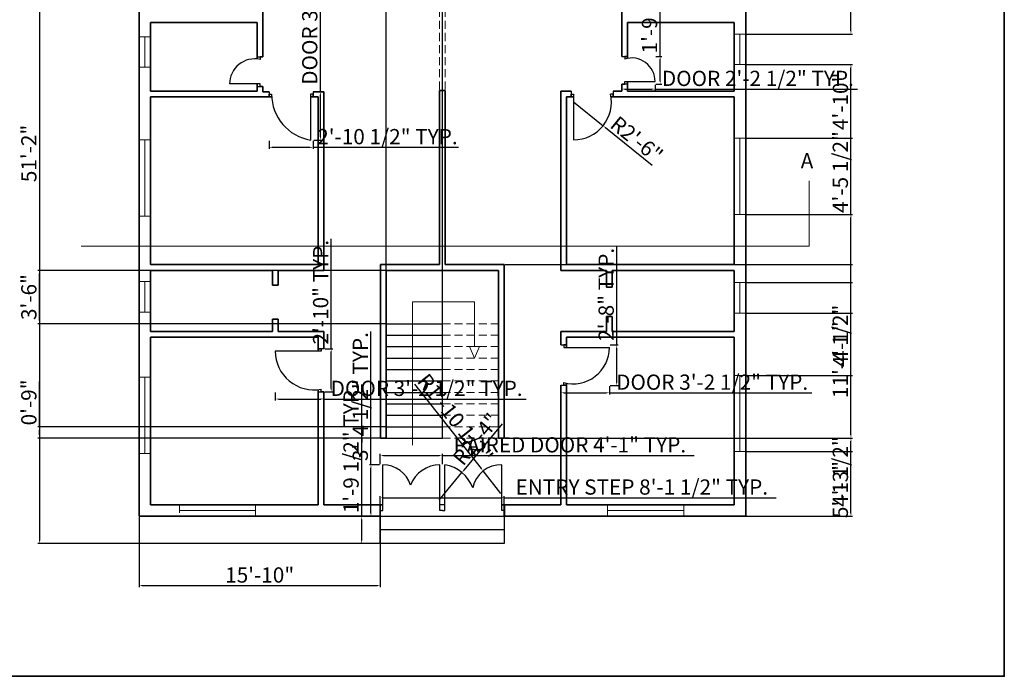
# Model space of a CAD drawing. Units: inches. Extents: x 2142 to 3604, y 1690 to 2981.
# Tile 5 of 9: x 2829 to 3604, y 1690 to 2207. Entities that reach past the tile are written whole.
import ezdxf

# ---------------------------------------------------------------- set-up
doc = ezdxf.new("R2010")
doc.units = ezdxf.units.IN
doc.linetypes.add('DASHED2', pattern=[9.525, 6.35, -3.175])
for name, color, linetype, lineweight in [('A-ANNO-DIMS', 2, 'Continuous', 18), ('A-ANNO-SYMB', 7, 'Continuous', 18), ('A-ANNO-TTLB', 7, 'Continuous', 35), ('A-DOOR', 4, 'Continuous', 25), ('A-FLOR-STRS', 7, 'Continuous', 25), ('A-FLOR-STRS-OVHD', 254, 'DASHED2', 18), ('A-GLAZ', 4, 'Continuous', 18), ('A-GLAZ-HIDN', 254, 'DASHED2', 18), ('A-WALL', 7, 'Continuous', 35), ('A-WALL-OVHD', 254, 'DASHED2', 18)]:
    doc.layers.add(name, color=color, linetype=linetype, lineweight=lineweight)
doc.styles.get("Standard").update_dxf_attribs({"font": 'arial.ttf'})
doc.dimstyles.new('ISO-25', dxfattribs={"dimtxt": 12, "dimasz": 2.5, "dimexe": 1.25, "dimexo": 0.625, "dimtad": 1, "dimdec": 0, "dimlunit": 3, "dimtxsty": 'Standard', "dimcen": 2.5, "dimadec": 0, "dimazin": 0, "dimtfac": 1, "dimtdec": 0, "dimtmove": 0, "dimatfit": 3, "dimfxl": 1, "dimarcsym": 0})

# ---------------------------------------------------------------- blocks, each defined once
blk = doc.blocks.new('DOOR-BATH-FRONT-R')
for p, q in [((0, 21.72), (4.5, 21.72)), ((4.5, 21.72), (2.25, 21.72)), ((2.25, 21.72), (2.25, 19.72)), ((4.5, 0), (0, 0)), ((0, 0), (2.25, 0)), ((2.25, 0), (2.25, 2)), ((2.25, 2), (26.25, 2))]:
    blk.add_line(p, q)
blk.add_arc((7.71, 2), 18.54, 0, 107.12458)
blk = doc.blocks.new('DOOR-BED-MID-R')
for p, q in [((0, 38.25), (0, 33.75)), ((0, 33.75), (0, 36)), ((0, 36), (2, 36)), ((2, 36), (2, 0)), ((33.13, 36), (31.13, 36)), ((33.13, 38.25), (33.13, 33.75)), ((33.13, 33.75), (33.13, 36))]:
    blk.add_line(p, q)
blk.add_arc((2, 29.79), 29.79, 270, 12.03684)
blk = doc.blocks.new('DOOR-BATH-FRONT-L')
for p, q in [((21.75, 23.31), (26.25, 23.31)), ((26.25, 23.31), (24, 23.31)), ((24, 23.31), (24, 21.31)), ((24, 2), (0, 2)), ((24, 0), (24, 2)), ((21.75, 0), (26.25, 0)), ((26.25, 0), (24, 0))]:
    blk.add_line(p, q)
blk.add_arc((19.77, 2), 19.77, 77.63852, 180)
blk = doc.blocks.new('DOOR-BED-FRONT-R')
for p, q in [((0, 31.64), (4.5, 31.64)), ((4.5, 31.64), (2.25, 31.64)), ((2.25, 31.64), (2.25, 29.64)), ((2.25, 29.64), (38.25, 29.64)), ((2.25, 0), (2.25, 2)), ((0, 0), (4.5, 0)), ((4.5, 0), (2.25, 0))]:
    blk.add_line(p, q)
blk.add_arc((9.64, 29.64), 28.61, 255.03948, 0)
blk = doc.blocks.new('DOOR-BED-FRONT-L')
for p, q in [((36, 31.84), (0, 31.84)), ((38.25, 33.84), (33.75, 33.84)), ((33.75, 33.84), (36, 33.84)), ((36, 33.84), (36, 31.84)), ((33.75, 0), (38.25, 0)), ((36, 0), (36, 2)), ((38.25, 0), (36, 0))]:
    blk.add_line(p, q)
blk.add_arc((30.37, 31.84), 30.37, 180, 280.68489)
blk = doc.blocks.new('DOOR-BED-MID-L')
for p, q in [((0, 38.05), (0, 33.95)), ((0, 33.95), (0, 36)), ((0, 36), (2, 36)), ((34.72, 36), (32.72, 36)), ((32.72, 36), (32.72, 0)), ((34.72, 38.05), (34.72, 38.05)), ((34.72, 38.05), (34.72, 33.95)), ((34.72, 33.95), (34.72, 36))]:
    blk.add_line(p, q)
blk.add_arc((38.45, 36), 36.45, 180, 260.94416)
blk = doc.blocks.new('DOOR-ENTRY-PAIR-L')
for p, q in [((2, 4.5), (2, 40.5)), ((46.88, 4.5), (46.88, 40.5)), ((0, 9), (0, 0)), ((0, 4.5), (2, 4.5)), ((48.88, 4.5), (46.88, 4.5))]:
    blk.add_line(p, q)
for centre, radius, start, end in [((2, 17.55), 22.95, 17.70587, 90), ((46.88, 15.91), 24.59, 90, 159.47898)]:
    blk.add_arc(centre, radius, start, end)
blk = doc.blocks.new('DOOR-ENTRY-PAIR-R')
for p, q in [((2, 4.5), (2, 40.5)), ((46.89, 4.5), (46.89, 40.5)), ((48.89, 9), (48.89, 0)), ((0, 4.5), (2, 4.5)), ((48.89, 4.5), (46.89, 4.5)), ((48.89, 0), (48.89, 4.5))]:
    blk.add_line(p, q)
for centre, radius, start, end in [((-2.51, 12.76), 28.1, 19.96217, 80.77047), ((46.01, 17.98), 22.54, 87.78446, 168.79388)]:
    blk.add_arc(centre, radius, start, end)
blk = doc.blocks.new('STEP-ENTRY')
blk.add_line((97.55, 10.76), (0, 10.76))
blk.add_lwpolyline([(0, 21.52), (97.55, 21.52), (97.55, 0), (0, 0)], close=True)
blk = doc.blocks.new('WINDOW-60')
for p, q in [((0, 60), (9, 60)), ((9, 60), (4.5, 60)), ((4.5, 60), (4.5, 0)), ((4.5, 0), (0, 0)), ((0, 0), (9, 0))]:
    blk.add_line(p, q)
blk = doc.blocks.new('WINDOW-24')
for p, q in [((0, 24), (9, 24)), ((9, 24), (4.5, 24)), ((4.5, 24), (4.5, 0)), ((4.5, 0), (0, 0)), ((0, 0), (9, 0))]:
    blk.add_line(p, q)
blk = doc.blocks.new('WINDOW-60-ENTRY')
for p, q in [((60, 4.5), (60, 9)), ((60, 9), (60, 0)), ((0, 4.5), (60, 4.5))]:
    blk.add_line(p, q)
blk = doc.blocks.new('STAIR-RETURN-ARROW')
for p, q in [((0, 0), (0, 112.66)), ((0, 112.66), (48.8, 112.66)), ((48.8, 112.66), (48.8, 77.43)), ((52.73, 77.43), (44.99, 77.43)), ((44.99, 77.43), (48.8, 68.43)), ((48.8, 68.43), (52.73, 77.43)), ((48.8, 68.43), (48.8, 68.43))]:
    blk.add_line(p, q)
blk = doc.blocks.new('*D53')
at = {"layer": 'A-ANNO-DIMS', "color": 0, "lineweight": -2, "transparency": 16777216}
for p, q in [((3303.33, 2155.54), (3303.33, 2150.98)), ((3329.58, 2155.54), (3329.58, 2150.98)), ((3305.83, 2152.23), (3327.08, 2152.23)), ((3329.58, 2152.23), (3488.79, 2152.23))]:
    blk.add_line(p, q, dxfattribs=at)
at = {"layer": 'A-ANNO-DIMS', "color": 0, "transparency": 16777216}
for points in [[(3305.83, 2152.64), (3305.83, 2151.81), (3303.33, 2152.23)], [(3327.08, 2152.64), (3327.08, 2151.81), (3329.58, 2152.23)]]:
    blk.add_solid(points, dxfattribs=at)
at = {"layer": 'Defpoints', "color": 0, "transparency": 16777216}
for p in [(3303.33, 2156.16), (3329.58, 2156.16), (3329.58, 2152.23)]:
    blk.add_point(p, dxfattribs=at)
at = {"layer": 'A-ANNO-DIMS', "color": 0, "transparency": 16777216, "insert": (3410.44, 2159.06), "char_height": 12, "attachment_point": 5}
blk.add_mtext('DOOR 2\'-2 1/2" TYP.', dxfattribs=at)
blk = doc.blocks.new('*D54')
at = {"layer": 'A-ANNO-DIMS', "color": 0, "lineweight": -2, "transparency": 16777216}
for p, q in [((3333.52, 2177.88), (3333.52, 2281.61)), ((3330.21, 2177.88), (3334.77, 2177.88)), ((3333.52, 2158.66), (3333.52, 2175.38)), ((3330.21, 2156.16), (3334.77, 2156.16))]:
    blk.add_line(p, q, dxfattribs=at)
at = {"layer": 'A-ANNO-DIMS', "color": 0, "transparency": 16777216}
for points in [[(3333.1, 2175.38), (3333.94, 2175.38), (3333.52, 2177.88)], [(3333.1, 2158.66), (3333.94, 2158.66), (3333.52, 2156.16)]]:
    blk.add_solid(points, dxfattribs=at)
at = {"layer": 'Defpoints', "color": 0, "transparency": 16777216}
for p in [(3329.58, 2177.88), (3333.52, 2177.88), (3329.58, 2156.16)]:
    blk.add_point(p, dxfattribs=at)
at = {"layer": 'A-ANNO-DIMS', "color": 0, "transparency": 16777216, "insert": (3326.69, 2231), "char_height": 12, "attachment_point": 5, "rotation": 90}
blk.add_mtext('1\'-9 1/2" TYP.', dxfattribs=at)
blk = doc.blocks.new('*D55')
at = {"layer": 'A-ANNO-DIMS', "color": 0, "lineweight": -2, "transparency": 16777216}
for p, q in [((3066.08, 2150.15), (3066.08, 2281.4)), ((3061, 2150.15), (3067.33, 2150.15)), ((3066.08, 2114.61), (3066.08, 2147.65)), ((3061, 2112.11), (3067.33, 2112.11))]:
    blk.add_line(p, q, dxfattribs=at)
at = {"layer": 'A-ANNO-DIMS', "color": 0, "transparency": 16777216}
for points in [[(3065.66, 2147.65), (3066.5, 2147.65), (3066.08, 2150.15)], [(3065.66, 2114.61), (3066.5, 2114.61), (3066.08, 2112.11)]]:
    blk.add_solid(points, dxfattribs=at)
at = {"layer": 'Defpoints', "color": 0, "transparency": 16777216}
for p in [(3060.37, 2150.15), (3066.08, 2150.15), (3060.37, 2112.11)]:
    blk.add_point(p, dxfattribs=at)
at = {"layer": 'A-ANNO-DIMS', "color": 0, "transparency": 16777216, "insert": (3059.24, 2217.03), "char_height": 12, "attachment_point": 5, "rotation": 90}
blk.add_mtext('DOOR 3\'-2" TYP.', dxfattribs=at)
blk = doc.blocks.new('*D56')
at = {"layer": 'A-ANNO-DIMS', "color": 0, "lineweight": -2, "transparency": 16777216}
for p, q in [((3025.66, 2111.48), (3025.66, 2105.15)), ((3060.37, 2111.48), (3060.37, 2105.15)), ((3028.16, 2106.4), (3057.87, 2106.4)), ((3060.37, 2106.4), (3174.76, 2106.4))]:
    blk.add_line(p, q, dxfattribs=at)
at = {"layer": 'A-ANNO-DIMS', "color": 0, "transparency": 16777216}
for points in [[(3028.16, 2106.82), (3028.16, 2105.98), (3025.66, 2106.4)], [(3057.87, 2106.82), (3057.87, 2105.98), (3060.37, 2106.4)]]:
    blk.add_solid(points, dxfattribs=at)
at = {"layer": 'Defpoints', "color": 0, "transparency": 16777216}
for p in [(3025.66, 2112.11), (3060.37, 2112.11), (3060.37, 2106.4)]:
    blk.add_point(p, dxfattribs=at)
at = {"layer": 'A-ANNO-DIMS', "color": 0, "transparency": 16777216, "insert": (3118.82, 2113.23), "char_height": 12, "attachment_point": 5}
blk.add_mtext('2\'-10 1/2" TYP.', dxfattribs=at)
blk = doc.blocks.new('*D59')
at = {"layer": 'A-ANNO-DIMS', "color": 0, "lineweight": -2, "transparency": 16777216}
for p, q in [((3030.58, 1913.44), (3030.58, 1907.08)), ((3033.08, 1908.33), (3066.33, 1908.33)), ((3068.83, 1913.44), (3068.83, 1907.08)), ((3068.83, 1908.33), (3228.04, 1908.33))]:
    blk.add_line(p, q, dxfattribs=at)
at = {"layer": 'A-ANNO-DIMS', "color": 0, "transparency": 16777216}
for points in [[(3033.08, 1908.75), (3033.08, 1907.91), (3030.58, 1908.33)], [(3066.33, 1908.75), (3066.33, 1907.91), (3068.83, 1908.33)]]:
    blk.add_solid(points, dxfattribs=at)
at = {"layer": 'Defpoints', "color": 0, "transparency": 16777216}
for p in [(3030.58, 1914.07), (3068.83, 1914.07), (3068.83, 1908.33)]:
    blk.add_point(p, dxfattribs=at)
at = {"layer": 'A-ANNO-DIMS', "color": 0, "transparency": 16777216, "insert": (3149.69, 1915.17), "char_height": 12, "attachment_point": 5}
blk.add_mtext('DOOR 3\'-2 1/2" TYP.', dxfattribs=at)
blk = doc.blocks.new('*D60')
at = {"layer": 'A-ANNO-DIMS', "color": 0, "lineweight": -2, "transparency": 16777216}
for p, q in [((3074.57, 1947.91), (3074.57, 2034.33)), ((3069.46, 1947.91), (3075.82, 1947.91)), ((3074.57, 1916.57), (3074.57, 1945.41)), ((3069.46, 1914.07), (3075.82, 1914.07))]:
    blk.add_line(p, q, dxfattribs=at)
at = {"layer": 'A-ANNO-DIMS', "color": 0, "transparency": 16777216}
for points in [[(3074.15, 1945.41), (3074.99, 1945.41), (3074.57, 1947.91)], [(3074.15, 1916.57), (3074.99, 1916.57), (3074.57, 1914.07)]]:
    blk.add_solid(points, dxfattribs=at)
at = {"layer": 'Defpoints', "color": 0, "transparency": 16777216}
for p in [(3068.83, 1947.91), (3074.57, 1947.91), (3068.83, 1914.07)]:
    blk.add_point(p, dxfattribs=at)
at = {"layer": 'A-ANNO-DIMS', "color": 0, "transparency": 16777216, "insert": (3067.82, 1992.37), "char_height": 12, "attachment_point": 5, "rotation": 90}
blk.add_mtext('2\'-10" TYP.', dxfattribs=at)
blk = doc.blocks.new('*D61')
at = {"layer": 'A-ANNO-DIMS', "color": 0, "lineweight": -2, "transparency": 16777216}
for p, q in [((3255.33, 1918.32), (3255.33, 1911.95)), ((3293.58, 1918.32), (3293.58, 1911.95)), ((3257.83, 1913.2), (3291.08, 1913.2)), ((3293.58, 1913.2), (3452.79, 1913.2))]:
    blk.add_line(p, q, dxfattribs=at)
at = {"layer": 'A-ANNO-DIMS', "color": 0, "transparency": 16777216}
for points in [[(3257.83, 1913.62), (3257.83, 1912.79), (3255.33, 1913.2)], [(3291.08, 1913.62), (3291.08, 1912.79), (3293.58, 1913.2)]]:
    blk.add_solid(points, dxfattribs=at)
at = {"layer": 'Defpoints', "color": 0, "transparency": 16777216}
for p in [(3255.33, 1918.94), (3293.58, 1918.94), (3293.58, 1913.2)]:
    blk.add_point(p, dxfattribs=at)
at = {"layer": 'A-ANNO-DIMS', "color": 0, "transparency": 16777216, "insert": (3374.44, 1920.04), "char_height": 12, "attachment_point": 5}
blk.add_mtext('DOOR 3\'-2 1/2" TYP.', dxfattribs=at)
blk = doc.blocks.new('*D62')
at = {"layer": 'A-ANNO-DIMS', "color": 0, "lineweight": -2, "transparency": 16777216}
for p, q in [((3299.32, 1950.88), (3299.32, 2027.98)), ((3294.21, 1950.88), (3300.57, 1950.88)), ((3299.32, 1921.44), (3299.32, 1948.38)), ((3294.21, 1918.94), (3300.57, 1918.94))]:
    blk.add_line(p, q, dxfattribs=at)
at = {"layer": 'A-ANNO-DIMS', "color": 0, "transparency": 16777216}
for points in [[(3298.9, 1948.38), (3299.74, 1948.38), (3299.32, 1950.88)], [(3298.9, 1921.44), (3299.74, 1921.44), (3299.32, 1918.94)]]:
    blk.add_solid(points, dxfattribs=at)
at = {"layer": 'Defpoints', "color": 0, "transparency": 16777216}
for p in [(3293.58, 1950.88), (3299.32, 1950.88), (3293.58, 1918.94)]:
    blk.add_point(p, dxfattribs=at)
at = {"layer": 'A-ANNO-DIMS', "color": 0, "transparency": 16777216, "insert": (3292.57, 1990.68), "char_height": 12, "attachment_point": 5, "rotation": 90}
blk.add_mtext('2\'-8" TYP.', dxfattribs=at)
blk = doc.blocks.new('*D63')
at = {"layer": 'A-ANNO-DIMS', "color": 0, "lineweight": -2, "transparency": 16777216}
for p, q in [((3113.2, 1857.18), (3113.2, 1865.14)), ((3115.7, 1863.89), (3159.58, 1863.89)), ((3162.08, 1857.18), (3162.08, 1865.14)), ((3162.08, 1863.89), (3360.4, 1863.89))]:
    blk.add_line(p, q, dxfattribs=at)
at = {"layer": 'A-ANNO-DIMS', "color": 0, "transparency": 16777216}
for points in [[(3115.7, 1864.31), (3115.7, 1863.47), (3113.2, 1863.89)], [(3159.58, 1864.31), (3159.58, 1863.47), (3162.08, 1863.89)]]:
    blk.add_solid(points, dxfattribs=at)
at = {"layer": 'Defpoints', "color": 0, "transparency": 16777216}
for p in [(3162.08, 1863.89), (3113.2, 1856.56), (3162.08, 1856.56)]:
    blk.add_point(p, dxfattribs=at)
at = {"layer": 'A-ANNO-DIMS', "color": 0, "transparency": 16777216, "insert": (3262.49, 1870.72), "char_height": 12, "attachment_point": 5}
blk.add_mtext('PAIRED DOOR 4\'-1" TYP.', dxfattribs=at)
blk = doc.blocks.new('*D64')
at = {"layer": 'A-ANNO-DIMS', "color": 0, "lineweight": -2, "transparency": 16777216}
for p, q in [((3105.87, 1856.56), (3105.87, 1961.41)), ((3112.57, 1856.56), (3104.62, 1856.56)), ((3105.87, 1818.56), (3105.87, 1854.06)), ((3112.57, 1816.06), (3104.62, 1816.06))]:
    blk.add_line(p, q, dxfattribs=at)
at = {"layer": 'A-ANNO-DIMS', "color": 0, "transparency": 16777216}
for points in [[(3105.45, 1854.06), (3106.28, 1854.06), (3105.87, 1856.56)], [(3105.45, 1818.56), (3106.28, 1818.56), (3105.87, 1816.06)]]:
    blk.add_solid(points, dxfattribs=at)
at = {"layer": 'Defpoints', "color": 0, "transparency": 16777216}
for p in [(3105.87, 1856.56), (3113.2, 1856.56), (3113.2, 1816.06)]:
    blk.add_point(p, dxfattribs=at)
at = {"layer": 'A-ANNO-DIMS', "color": 0, "transparency": 16777216, "insert": (3099.03, 1910.23), "char_height": 12, "attachment_point": 5, "rotation": 90}
blk.add_mtext('3\'-4 1/2" TYP.', dxfattribs=at)
blk = doc.blocks.new('*D71')
at = {"layer": 'A-ANNO-DIMS', "color": 0, "lineweight": -2, "transparency": 16777216}
for p, q in [((3113.2, 1816.68), (3113.2, 1831.94)), ((3115.7, 1830.69), (3208.25, 1830.69)), ((3210.75, 1816.68), (3210.75, 1831.94)), ((3210.75, 1830.69), (3424.89, 1830.69))]:
    blk.add_line(p, q, dxfattribs=at)
at = {"layer": 'A-ANNO-DIMS', "color": 0, "transparency": 16777216}
for points in [[(3115.7, 1831.11), (3115.7, 1830.27), (3113.2, 1830.69)], [(3208.25, 1831.11), (3208.25, 1830.27), (3210.75, 1830.69)]]:
    blk.add_solid(points, dxfattribs=at)
at = {"layer": 'Defpoints', "color": 0, "transparency": 16777216}
for p in [(3210.75, 1830.69), (3113.2, 1816.06), (3210.75, 1816.06)]:
    blk.add_point(p, dxfattribs=at)
at = {"layer": 'A-ANNO-DIMS', "color": 0, "transparency": 16777216, "insert": (3319.07, 1837.52), "char_height": 12, "attachment_point": 5}
blk.add_mtext('ENTRY STEP 8\'-1 1/2" TYP.', dxfattribs=at)
blk = doc.blocks.new('*D72')
at = {"layer": 'A-ANNO-DIMS', "color": 0, "lineweight": -2, "transparency": 16777216}
for p, q in [((3098.57, 1816.06), (3098.57, 1919.79)), ((3112.57, 1816.06), (3097.32, 1816.06)), ((3098.57, 1797.04), (3098.57, 1813.56)), ((3112.57, 1794.54), (3097.32, 1794.54))]:
    blk.add_line(p, q, dxfattribs=at)
at = {"layer": 'A-ANNO-DIMS', "color": 0, "transparency": 16777216}
for points in [[(3098.15, 1813.56), (3098.98, 1813.56), (3098.57, 1816.06)], [(3098.15, 1797.04), (3098.98, 1797.04), (3098.57, 1794.54)]]:
    blk.add_solid(points, dxfattribs=at)
at = {"layer": 'Defpoints', "color": 0, "transparency": 16777216}
for p in [(3098.57, 1816.06), (3113.2, 1816.06), (3113.2, 1794.54)]:
    blk.add_point(p, dxfattribs=at)
at = {"layer": 'A-ANNO-DIMS', "color": 0, "transparency": 16777216, "insert": (3091.74, 1869.17), "char_height": 12, "attachment_point": 5, "rotation": 90}
blk.add_mtext('1\'-9 1/2" TYP.', dxfattribs=at)
blk = doc.blocks.new('*D78')
at = {"layer": 'A-ANNO-DIMS', "color": 0, "lineweight": -2, "transparency": 16777216}
for p, q in [((2922.71, 2408.56), (2843.63, 2408.56)), ((2844.88, 2406.06), (2844.88, 1797.04)), ((3112.57, 1794.54), (2843.63, 1794.54))]:
    blk.add_line(p, q, dxfattribs=at)
at = {"layer": 'A-ANNO-DIMS', "color": 0, "transparency": 16777216}
for points in [[(2844.46, 2406.06), (2845.3, 2406.06), (2844.88, 2408.56)], [(2844.46, 1797.04), (2845.3, 1797.04), (2844.88, 1794.54)]]:
    blk.add_solid(points, dxfattribs=at)
at = {"layer": 'Defpoints', "color": 0, "transparency": 16777216}
for p in [(2923.33, 2408.56), (2844.88, 1794.54), (3113.2, 1794.54)]:
    blk.add_point(p, dxfattribs=at)
at = {"layer": 'A-ANNO-DIMS', "color": 0, "transparency": 16777216, "insert": (2838.13, 2101.55), "char_height": 12, "attachment_point": 5, "rotation": 90}
blk.add_mtext('51\'-2"', dxfattribs=at)
blk = doc.blocks.new('*D110')
at = {"layer": 'A-ANNO-DIMS', "color": 0, "lineweight": -2, "transparency": 16777216}
for p, q in [((3211.46, 2014.06), (3484.95, 2014.06)), ((3483.7, 1880.06), (3483.7, 2011.56)), ((3211.46, 1877.56), (3484.95, 1877.56))]:
    blk.add_line(p, q, dxfattribs=at)
at = {"layer": 'A-ANNO-DIMS', "color": 0, "transparency": 16777216}
for points in [[(3483.29, 2011.56), (3484.12, 2011.56), (3483.7, 2014.06)], [(3483.29, 1880.06), (3484.12, 1880.06), (3483.7, 1877.56)]]:
    blk.add_solid(points, dxfattribs=at)
at = {"layer": 'Defpoints', "color": 0, "transparency": 16777216}
for p in [(3210.83, 2014.06), (3483.7, 2014.06), (3210.83, 1877.56)]:
    blk.add_point(p, dxfattribs=at)
at = {"layer": 'A-ANNO-DIMS', "color": 0, "transparency": 16777216, "insert": (3476.88, 1945.81), "char_height": 12, "attachment_point": 5, "rotation": 90}
blk.add_mtext('11\'-4 1/2"', dxfattribs=at)
blk = doc.blocks.new('*D111')
at = {"layer": 'A-ANNO-DIMS', "color": 0, "lineweight": -2, "transparency": 16777216}
for p, q in [((3211.46, 1877.56), (3484.95, 1877.56)), ((3483.7, 1818.56), (3483.7, 1875.06)), ((3211.37, 1816.06), (3484.95, 1816.06))]:
    blk.add_line(p, q, dxfattribs=at)
at = {"layer": 'A-ANNO-DIMS', "color": 0, "transparency": 16777216}
for points in [[(3483.29, 1875.06), (3484.12, 1875.06), (3483.7, 1877.56)], [(3483.29, 1818.56), (3484.12, 1818.56), (3483.7, 1816.06)]]:
    blk.add_solid(points, dxfattribs=at)
at = {"layer": 'Defpoints', "color": 0, "transparency": 16777216}
for p in [(3210.83, 1877.56), (3483.7, 1877.56), (3210.75, 1816.06)]:
    blk.add_point(p, dxfattribs=at)
at = {"layer": 'A-ANNO-DIMS', "color": 0, "transparency": 16777216, "insert": (3476.88, 1846.81), "char_height": 12, "attachment_point": 5, "rotation": 90}
blk.add_mtext('5\'-1 1/2"', dxfattribs=at)
blk = doc.blocks.new('*D112')
at = {"layer": 'A-ANNO-DIMS', "color": 0, "lineweight": -2, "transparency": 16777216}
for p, q in [((3117.83, 1878.18), (3117.83, 2442.81)), ((3120.33, 2441.56), (3159.58, 2441.56)), ((3162.08, 1878.18), (3162.08, 2442.81)), ((3162.08, 2441.56), (3225.69, 2441.56))]:
    blk.add_line(p, q, dxfattribs=at)
at = {"layer": 'A-ANNO-DIMS', "color": 0, "transparency": 16777216}
for points in [[(3120.33, 2441.98), (3120.33, 2441.14), (3117.83, 2441.56)], [(3159.58, 2441.98), (3159.58, 2441.14), (3162.08, 2441.56)]]:
    blk.add_solid(points, dxfattribs=at)
at = {"layer": 'Defpoints', "color": 0, "transparency": 16777216}
for p in [(3162.08, 2441.56), (3117.83, 1877.56), (3162.08, 1877.56)]:
    blk.add_point(p, dxfattribs=at)
at = {"layer": 'A-ANNO-DIMS', "color": 0, "transparency": 16777216, "insert": (3195.13, 2448.39), "char_height": 12, "attachment_point": 5}
blk.add_mtext('3\'-8 1/2"', dxfattribs=at)
blk = doc.blocks.new('*D113')
at = {"layer": 'A-ANNO-DIMS', "color": 0, "lineweight": -2, "transparency": 16777216}
for p, q in [((2844.88, 1886.56), (2844.88, 1922.21)), ((3117.21, 1886.56), (2843.63, 1886.56)), ((2844.88, 1880.06), (2844.88, 1884.06)), ((3117.21, 1877.56), (2843.63, 1877.56))]:
    blk.add_line(p, q, dxfattribs=at)
at = {"layer": 'A-ANNO-DIMS', "color": 0, "transparency": 16777216}
for points in [[(2844.46, 1884.06), (2845.3, 1884.06), (2844.88, 1886.56)], [(2844.46, 1880.06), (2845.3, 1880.06), (2844.88, 1877.56)]]:
    blk.add_solid(points, dxfattribs=at)
at = {"layer": 'Defpoints', "color": 0, "transparency": 16777216}
for p in [(2844.88, 1886.56), (3117.83, 1886.56), (3117.83, 1877.56)]:
    blk.add_point(p, dxfattribs=at)
at = {"layer": 'A-ANNO-DIMS', "color": 0, "transparency": 16777216, "insert": (2838.13, 1905.63), "char_height": 12, "attachment_point": 5, "rotation": 90}
blk.add_mtext('0\'-9"', dxfattribs=at)
blk = doc.blocks.new('*D114')
at = {"layer": 'A-ANNO-DIMS', "color": 0, "lineweight": -2, "transparency": 16777216}
for p, q in [((3117.21, 2009.56), (2843.63, 2009.56)), ((2844.88, 1970.06), (2844.88, 2007.06)), ((3117.21, 1967.56), (2843.63, 1967.56))]:
    blk.add_line(p, q, dxfattribs=at)
at = {"layer": 'A-ANNO-DIMS', "color": 0, "transparency": 16777216}
for points in [[(2844.46, 2007.06), (2845.3, 2007.06), (2844.88, 2009.56)], [(2844.46, 1970.06), (2845.3, 1970.06), (2844.88, 1967.56)]]:
    blk.add_solid(points, dxfattribs=at)
at = {"layer": 'Defpoints', "color": 0, "transparency": 16777216}
for p in [(2844.88, 2009.56), (3117.83, 2009.56), (3117.83, 1967.56)]:
    blk.add_point(p, dxfattribs=at)
at = {"layer": 'A-ANNO-DIMS', "color": 0, "transparency": 16777216, "insert": (2838.12, 1988.56), "char_height": 12, "attachment_point": 5, "rotation": 90}
blk.add_mtext('3\'-6"', dxfattribs=at)
blk = doc.blocks.new('*D115')
at = {"layer": 'A-ANNO-DIMS', "color": 0, "lineweight": -2, "transparency": 16777216}
for p, q in [((2923.33, 1815.43), (2923.33, 1760.29)), ((3113.2, 1815.43), (3113.2, 1760.29)), ((2925.83, 1761.54), (3110.7, 1761.54))]:
    blk.add_line(p, q, dxfattribs=at)
at = {"layer": 'A-ANNO-DIMS', "color": 0, "transparency": 16777216}
for points in [[(2925.83, 1761.95), (2925.83, 1761.12), (2923.33, 1761.54)], [(3110.7, 1761.95), (3110.7, 1761.12), (3113.2, 1761.54)]]:
    blk.add_solid(points, dxfattribs=at)
at = {"layer": 'Defpoints', "color": 0, "transparency": 16777216}
for p in [(2923.33, 1816.06), (3113.2, 1816.06), (3113.2, 1761.54)]:
    blk.add_point(p, dxfattribs=at)
at = {"layer": 'A-ANNO-DIMS', "color": 0, "transparency": 16777216, "insert": (3018.27, 1768.29), "char_height": 12, "attachment_point": 5}
blk.add_mtext('15\'-10"', dxfattribs=at)
blk = doc.blocks.new('*D116')
at = {"layer": 'A-ANNO-DIMS', "color": 0, "lineweight": -2, "transparency": 16777216}
for p, q in [((3401.46, 1866.94), (3484.95, 1866.94)), ((3483.7, 1818.56), (3483.7, 1864.44)), ((3401.46, 1816.06), (3484.95, 1816.06))]:
    blk.add_line(p, q, dxfattribs=at)
at = {"layer": 'A-ANNO-DIMS', "color": 0, "transparency": 16777216}
for points in [[(3483.29, 1864.44), (3484.12, 1864.44), (3483.7, 1866.94)], [(3483.29, 1818.56), (3484.12, 1818.56), (3483.7, 1816.06)]]:
    blk.add_solid(points, dxfattribs=at)
at = {"layer": 'Defpoints', "color": 0, "transparency": 16777216}
for p in [(3400.83, 1866.94), (3483.7, 1866.94), (3400.83, 1816.06)]:
    blk.add_point(p, dxfattribs=at)
at = {"layer": 'A-ANNO-DIMS', "color": 0, "transparency": 16777216, "insert": (3476.95, 1841.5), "char_height": 12, "attachment_point": 5, "rotation": 90}
blk.add_mtext('4\'-3"', dxfattribs=at)
blk = doc.blocks.new('*D117')
at = {"layer": 'A-ANNO-DIMS', "color": 0, "lineweight": -2, "transparency": 16777216}
for p, q in [((3401.46, 1975.88), (3484.95, 1975.88)), ((3483.7, 1929.44), (3483.7, 1973.38)), ((3401.46, 1926.94), (3484.95, 1926.94))]:
    blk.add_line(p, q, dxfattribs=at)
at = {"layer": 'A-ANNO-DIMS', "color": 0, "transparency": 16777216}
for points in [[(3483.29, 1973.38), (3484.12, 1973.38), (3483.7, 1975.88)], [(3483.29, 1929.44), (3484.12, 1929.44), (3483.7, 1926.94)]]:
    blk.add_solid(points, dxfattribs=at)
at = {"layer": 'Defpoints', "color": 0, "transparency": 16777216}
for p in [(3400.83, 1975.88), (3483.7, 1975.88), (3400.83, 1926.94)]:
    blk.add_point(p, dxfattribs=at)
at = {"layer": 'A-ANNO-DIMS', "color": 0, "transparency": 16777216, "insert": (3477.06, 1951.41), "char_height": 12, "attachment_point": 5, "rotation": 90}
blk.add_mtext('4\'-1"', dxfattribs=at)
blk = doc.blocks.new('*D118')
at = {"layer": 'A-ANNO-DIMS', "color": 0, "lineweight": -2, "transparency": 16777216}
for p, q in [((3483.7, 2053.61), (3483.7, 2117.71)), ((3401.46, 2053.61), (3484.95, 2053.61)), ((3483.7, 2002.38), (3483.7, 2051.11)), ((3401.46, 1999.88), (3484.95, 1999.88))]:
    blk.add_line(p, q, dxfattribs=at)
at = {"layer": 'A-ANNO-DIMS', "color": 0, "transparency": 16777216}
for points in [[(3483.29, 2051.11), (3484.12, 2051.11), (3483.7, 2053.61)], [(3483.29, 2002.38), (3484.12, 2002.38), (3483.7, 1999.88)]]:
    blk.add_solid(points, dxfattribs=at)
at = {"layer": 'Defpoints', "color": 0, "transparency": 16777216}
for p in [(3400.83, 2053.61), (3483.7, 2053.61), (3400.83, 1999.88)]:
    blk.add_point(p, dxfattribs=at)
at = {"layer": 'A-ANNO-DIMS', "color": 0, "transparency": 16777216, "insert": (3476.88, 2086.91), "char_height": 12, "attachment_point": 5, "rotation": 90}
blk.add_mtext('4\'-5 1/2"', dxfattribs=at)
blk = doc.blocks.new('*D119')
at = {"layer": 'A-ANNO-DIMS', "color": 0, "lineweight": -2, "transparency": 16777216}
for p, q in [((3401.46, 2171.49), (3484.95, 2171.49)), ((3483.7, 2116.11), (3483.7, 2168.99)), ((3401.46, 2113.61), (3484.95, 2113.61))]:
    blk.add_line(p, q, dxfattribs=at)
at = {"layer": 'A-ANNO-DIMS', "color": 0, "transparency": 16777216}
for points in [[(3483.29, 2168.99), (3484.12, 2168.99), (3483.7, 2171.49)], [(3483.29, 2116.11), (3484.12, 2116.11), (3483.7, 2113.61)]]:
    blk.add_solid(points, dxfattribs=at)
at = {"layer": 'Defpoints', "color": 0, "transparency": 16777216}
for p in [(3400.83, 2171.49), (3483.7, 2171.49), (3400.83, 2113.61)]:
    blk.add_point(p, dxfattribs=at)
at = {"layer": 'A-ANNO-DIMS', "color": 0, "transparency": 16777216, "insert": (3476.95, 2142.55), "char_height": 12, "attachment_point": 5, "rotation": 90}
blk.add_mtext('4\'-10"', dxfattribs=at)
blk = doc.blocks.new('*D120')
at = {"layer": 'A-ANNO-DIMS', "color": 0, "lineweight": -2, "transparency": 16777216}
for p, q in [((3483.7, 2223.37), (3483.7, 2259.22)), ((3401.46, 2223.37), (3484.95, 2223.37)), ((3483.7, 2197.99), (3483.7, 2220.87)), ((3401.46, 2195.49), (3484.95, 2195.49))]:
    blk.add_line(p, q, dxfattribs=at)
at = {"layer": 'A-ANNO-DIMS', "color": 0, "transparency": 16777216}
for points in [[(3483.29, 2220.87), (3484.12, 2220.87), (3483.7, 2223.37)], [(3483.29, 2197.99), (3484.12, 2197.99), (3483.7, 2195.49)]]:
    blk.add_solid(points, dxfattribs=at)
at = {"layer": 'Defpoints', "color": 0, "transparency": 16777216}
for p in [(3400.83, 2223.37), (3483.7, 2223.37), (3400.83, 2195.49)]:
    blk.add_point(p, dxfattribs=at)
at = {"layer": 'A-ANNO-DIMS', "color": 0, "transparency": 16777216, "insert": (3477.06, 2242.54), "char_height": 12, "attachment_point": 5, "rotation": 90}
blk.add_mtext('2\'-4"', dxfattribs=at)
blk = doc.blocks.new('*D127')
at = {"layer": 'A-ANNO-DIMS', "color": 0, "lineweight": -2, "transparency": 16777216}
for p, q in [((3265.42, 2142.1), (3288.58, 2123.36)), ((3327.16, 2092.14), (3290.52, 2121.79))]:
    blk.add_line(p, q, dxfattribs=at)
at = {"layer": 'A-ANNO-DIMS', "color": 0, "transparency": 16777216}
blk.add_solid([(3290.78, 2122.11), (3290.26, 2121.46), (3288.58, 2123.36)], dxfattribs=at)
at = {"layer": 'Defpoints', "color": 0, "transparency": 16777216}
for p in [(3265.42, 2142.1), (3288.58, 2123.36)]:
    blk.add_point(p, dxfattribs=at)
at = {"layer": 'A-ANNO-DIMS', "color": 0, "transparency": 16777216, "insert": (3314.06, 2111.42), "char_height": 12, "attachment_point": 5, "rotation": 321.01899}
blk.add_mtext('R2\'-6"', dxfattribs=at)
blk = doc.blocks.new('*D129')
at = {"layer": 'A-ANNO-DIMS', "color": 0, "lineweight": -2, "transparency": 16777216}
for p, q in [((3209.16, 1888.69), (3179.09, 1852.39)), ((3159.58, 1828.82), (3177.5, 1850.46))]:
    blk.add_line(p, q, dxfattribs=at)
at = {"layer": 'A-ANNO-DIMS', "color": 0, "transparency": 16777216}
blk.add_solid([(3178.77, 1852.65), (3179.42, 1852.12), (3177.5, 1850.46)], dxfattribs=at)
at = {"layer": 'Defpoints', "color": 0, "transparency": 16777216}
for p in [(3177.5, 1850.46), (3159.58, 1828.82)]:
    blk.add_point(p, dxfattribs=at)
at = {"layer": 'A-ANNO-DIMS', "color": 0, "transparency": 16777216, "insert": (3189.8, 1875.74), "char_height": 12, "attachment_point": 5, "rotation": 50.36646}
blk.add_mtext('R2\'-4"', dxfattribs=at)
blk = doc.blocks.new('*D133')
at = {"layer": 'A-ANNO-DIMS', "color": 0, "lineweight": -2, "transparency": 16777216}
for p, q in [((3140.27, 1919.95), (3192.58, 1853.69)), ((3208.1, 1834.04), (3194.13, 1851.73))]:
    blk.add_line(p, q, dxfattribs=at)
at = {"layer": 'A-ANNO-DIMS', "color": 0, "transparency": 16777216}
blk.add_solid([(3192.91, 1853.95), (3192.26, 1853.43), (3194.13, 1851.73)], dxfattribs=at)
at = {"layer": 'Defpoints', "color": 0, "transparency": 16777216}
for p in [(3194.13, 1851.73), (3208.1, 1834.04)]:
    blk.add_point(p, dxfattribs=at)
at = {"layer": 'A-ANNO-DIMS', "color": 0, "transparency": 16777216, "insert": (3171.01, 1892.03), "char_height": 12, "attachment_point": 5, "rotation": 308.28965}
blk.add_mtext('R1\'-10 1/2"', dxfattribs=at)

msp = doc.modelspace()

# ---------------------------------------------------------------- linework, layer by layer
at = {"layer": 'A-ANNO-SYMB'}
for p, q in [((3450.7, 2028.72), (3450.7, 2079.98)), ((2877.88, 2028.72), (3450.7, 2028.72))]:
    msp.add_line(p, q, dxfattribs=at)
at = {"layer": 'A-ANNO-TTLB'}
msp.add_lwpolyline([(2142.1, 2981.01), (3604.42, 2981.01), (3604.42, 1690.13), (2142.1, 1690.13)], close=True, dxfattribs=at)
at = {"layer": 'A-DOOR'}
msp.add_line((3164.08, 1825.06), (3160.08, 1825.06), dxfattribs=at)
at = {"layer": 'A-FLOR-STRS'}
for p, q in [((3117.83, 1967.56), (3162.08, 1967.56)), ((3162.08, 1877.56), (3162.08, 1967.56)), ((3117.83, 1958.56), (3162.08, 1958.56)), ((3117.83, 1949.56), (3162.08, 1949.56)), ((3117.83, 1940.56), (3162.08, 1940.56)), ((3117.83, 1931.56), (3162.08, 1931.56)), ((3117.83, 1922.56), (3162.08, 1922.56)), ((3117.83, 1913.56), (3162.08, 1913.56)), ((3117.83, 1904.56), (3162.08, 1904.56)), ((3117.83, 1895.56), (3162.08, 1895.56)), ((3117.83, 1886.56), (3162.08, 1886.56)), ((3117.83, 1877.56), (3162.08, 1877.56))]:
    msp.add_line(p, q, dxfattribs=at)
at = {"layer": 'A-FLOR-STRS-OVHD'}
for p, q in [((3162.08, 1967.56), (3206.33, 1967.56)), ((3162.08, 1958.56), (3206.33, 1958.56)), ((3162.08, 1949.56), (3206.33, 1949.56)), ((3162.08, 1940.56), (3206.33, 1940.56)), ((3162.08, 1931.56), (3206.33, 1931.56)), ((3162.08, 1922.56), (3206.33, 1922.56)), ((3162.08, 1913.56), (3206.33, 1913.56)), ((3162.08, 1904.56), (3206.33, 1904.56)), ((3162.08, 1895.56), (3206.33, 1895.56)), ((3162.08, 1886.56), (3206.33, 1886.56)), ((3162.08, 1877.56), (3206.33, 1877.56))]:
    msp.add_line(p, q, dxfattribs=at)
at = {"layer": 'A-GLAZ-HIDN'}
msp.add_line((2955.1, 1825.06), (2955.1, 1816.06), dxfattribs=at)
at = {"layer": 'A-WALL'}
for p, q in [((2923.33, 2408.56), (2923.33, 1816.06)), ((3400.83, 2408.56), (3400.83, 1816.06)), ((3020.83, 2263.06), (3020.83, 2177.56)), ((3303.33, 2263.06), (3303.33, 2177.88)), ((2932.33, 2204.56), (3016.33, 2204.56)), ((2932.33, 2204.56), (2932.33, 2150.56)), ((3016.33, 2175.92), (3016.33, 2204.56)), ((3307.83, 2204.56), (3391.83, 2204.56)), ((3307.83, 2176.42), (3307.83, 2204.56)), ((3391.83, 2204.56), (3391.83, 2150.56)), ((3016.33, 2150.56), (3016.33, 2156.25)), ((3303.33, 2156.16), (3303.33, 2150.56)), ((3307.83, 2150.56), (3307.83, 2158.16)), ((2932.33, 2150.56), (3016.33, 2150.56)), ((3020.83, 2154.25), (3020.83, 2150.15)), ((3020.83, 2150.15), (3025.66, 2150.15)), ((3060.37, 2150.15), (3068.83, 2150.15)), ((3068.83, 2150.15), (3068.83, 2009.56)), ((3159.83, 2151.06), (3159.83, 2014.06)), ((3164.33, 2151.06), (3159.83, 2151.06)), ((3164.33, 2151.06), (3164.33, 2014.06)), ((3164.33, 2014.06), (3164.33, 2151.06)), ((3255.33, 2150.56), (3255.33, 2009.56)), ((3263.42, 2150.56), (3255.33, 2150.56)), ((3255.33, 2150.56), (3255.33, 2146.06)), ((3303.33, 2150.56), (3296.55, 2150.56)), ((3307.83, 2150.56), (3391.83, 2150.56)), ((2932.33, 2146.06), (3020.83, 2146.06)), ((2932.33, 2146.06), (2932.33, 2014.06)), ((2932.33, 2146.06), (3016.33, 2146.06)), ((3020.83, 2146.06), (3027.72, 2146.06)), ((3058.37, 2146.06), (3064.33, 2146.06)), ((3064.33, 2146.06), (3064.33, 2014.06)), ((3259.83, 2146.06), (3259.83, 2014.06)), ((3259.83, 2146.06), (3265.42, 2146.06)), ((3294.94, 2146.06), (3303.33, 2146.06)), ((3303.33, 2146.06), (3391.83, 2146.06)), ((3391.83, 2146.06), (3307.83, 2146.06)), ((3391.83, 2146.06), (3391.83, 2014.06)), ((2932.33, 2014.06), (3068.83, 2014.06)), ((2932.33, 2009.56), (2932.33, 1961.56)), ((2932.33, 2009.56), (3028.33, 2009.56)), ((3028.33, 1997.9), (3028.33, 2009.56)), ((3032.83, 2009.56), (3068.83, 2009.56)), ((3032.83, 1997.9), (3032.83, 2009.56)), ((3159.83, 2014.06), (3113.33, 2014.06)), ((3113.33, 1877.56), (3113.33, 2014.06)), ((3117.83, 2009.56), (3206.33, 2009.56)), ((3159.83, 2009.56), (3117.83, 2009.56)), ((3117.83, 2009.56), (3117.83, 1877.56)), ((3210.83, 2014.06), (3164.33, 2014.06)), ((3164.33, 2009.56), (3206.33, 2009.56)), ((3206.33, 2009.56), (3206.33, 1877.56)), ((3210.83, 1877.56), (3210.83, 2014.06)), ((3291.33, 2009.56), (3255.33, 2009.56)), ((3391.83, 2014.06), (3259.83, 2014.06)), ((3291.33, 2009.56), (3291.33, 1996.28)), ((3391.83, 2009.56), (3295.83, 2009.56)), ((3295.83, 1996.28), (3295.83, 2009.56)), ((3391.83, 2009.56), (3391.83, 1961.56)), ((3028.33, 1997.9), (3032.83, 1997.9)), ((3291.33, 1996.28), (3295.83, 1996.28)), ((3028.33, 1961.56), (3028.33, 1971.25)), ((3028.33, 1971.25), (3032.83, 1971.25)), ((3032.83, 1961.56), (3032.83, 1971.25)), ((3291.33, 1973.33), (3291.33, 1961.56)), ((3291.33, 1973.33), (3295.83, 1973.33)), ((3295.83, 1961.56), (3295.83, 1973.33)), ((2932.33, 1961.56), (3028.33, 1961.56)), ((3032.83, 1961.56), (3068.83, 1961.56)), ((3068.83, 1961.56), (3068.83, 1947.91)), ((3255.33, 1961.56), (3255.33, 1950.88)), ((3291.33, 1961.56), (3255.33, 1961.56)), ((3391.83, 1961.56), (3295.83, 1961.56)), ((3391.83, 1961.56), (3295.83, 1961.56)), ((2932.33, 1957.06), (2932.33, 1825.06)), ((2932.33, 1957.06), (3064.33, 1957.06)), ((2932.33, 1957.06), (3064.33, 1957.06)), ((3028.33, 1957.06), (3032.83, 1957.06)), ((3064.33, 1957.06), (3064.33, 1945.91)), ((3259.83, 1957.06), (3259.83, 1948.88)), ((3391.83, 1957.06), (3259.83, 1957.06)), ((3391.83, 1957.06), (3391.83, 1825.06)), ((3064.33, 1915.73), (3064.33, 1825.06)), ((3255.33, 1919.24), (3255.33, 1825.06)), ((3259.83, 1920.73), (3259.83, 1825.06)), ((3068.83, 1914.07), (3068.83, 1825.06)), ((3117.83, 1877.56), (3113.33, 1877.56)), ((3206.33, 1877.56), (3210.83, 1877.56)), ((3064.33, 1825.06), (2932.33, 1825.06)), ((3115.2, 1825.06), (3068.83, 1825.06)), ((3255.33, 1825.06), (3208.97, 1825.06)), ((3391.83, 1825.06), (3259.83, 1825.06)), ((3113.2, 1816.06), (2923.33, 1816.06)), ((3400.83, 1816.06), (3210.97, 1816.06))]:
    msp.add_line(p, q, dxfattribs=at)
at = {"layer": 'A-WALL-OVHD'}
for p, q in [((3159.83, 2263.06), (3159.83, 2151.06)), ((3164.33, 2263.06), (3164.33, 2151.06))]:
    msp.add_line(p, q, dxfattribs=at)

# ---------------------------------------------------------------- block references
at = {"layer": 'A-ANNO-SYMB'}
msp.add_blockref('STAIR-RETURN-ARROW', (3138.45, 1872.13), dxfattribs=at)
at = {"layer": 'A-DOOR'}
for name, p in [('DOOR-BATH-FRONT-L', (2994.58, 2154.25)), ('DOOR-BATH-FRONT-R', (3303.33, 2156.16)), ('DOOR-BED-MID-L', (3025.66, 2112.11)), ('DOOR-BED-MID-R', (3263.42, 2112.31)), ('DOOR-BED-FRONT-L', (3030.58, 1914.07)), ('DOOR-BED-FRONT-R', (3255.33, 1919.24)), ('DOOR-ENTRY-PAIR-L', (3113.2, 1816.06)), ('DOOR-ENTRY-PAIR-R', (3162.08, 1816.06))]:
    msp.add_blockref(name, p, dxfattribs=at)
at = {"layer": 'A-FLOR-STRS'}
msp.add_blockref('STEP-ENTRY', (3113.2, 1794.54), dxfattribs=at)
at = {"layer": 'A-GLAZ'}
for name, p in [('WINDOW-24', (2923.33, 2169.41)), ('WINDOW-24', (3391.83, 2171.49)), ('WINDOW-60', (2923.33, 2052.31)), ('WINDOW-60', (3391.83, 2053.62)), ('WINDOW-24', (2923.33, 1976.69)), ('WINDOW-24', (3391.83, 1975.88)), ('WINDOW-60', (2923.33, 1865.5)), ('WINDOW-60', (3391.83, 1866.94)), ('WINDOW-60-ENTRY', (2955.1, 1816.06))]:
    msp.add_blockref(name, p, dxfattribs=at)
at = {"layer": 'A-GLAZ', "extrusion": (0, 0, -1), "zscale": -1, "rotation": 270}
msp.add_blockref('WINDOW-60', (-3352.11, 1825.06), dxfattribs=at)

# ---------------------------------------------------------------- texts
at = {"layer": 'A-ANNO-SYMB', "insert": (3444.13, 2101.79), "char_height": 12, "attachment_point": 1}
msp.add_mtext_dynamic_manual_height_columns('A', width=44.3478, gutter_width=12.5, heights=[0], dxfattribs=at)

# ---------------------------------------------------------------- dimensions: what is measured, and where the dimension line sits
at = {"layer": 'A-ANNO-DIMS'}
for base, p1, p2, picture, middle in [((3162.083094, 2441.558519), (3117.833094, 1877.558519), (3162.083094, 1877.558519), '*D112', (3195.13442415, 2448.39225024)), ((3113.2, 1761.54), (2923.33, 1816.06), (3113.2, 1816.06), '*D115', (3018.27, 1768.29))]:
    dim = msp.add_linear_dim(base=base, p1=p1, p2=p2, dimstyle='ISO-25', override={"dimdec": 1, "dimlfac": 1, "dimrnd": 0, "dimzin": 1, "dimdsep": 46, "dimlunit": 4, "dimfrac": 2}, dxfattribs=at)
    dim.commit()
    dim.dimension.update_dxf_attribs({"geometry": picture, "text_midpoint": middle})
for base, p1, p2, picture, middle in [((2844.88, 1794.54), (2923.33, 2408.56), (3113.2, 1794.54), '*D78', (2838.13, 2101.55)), ((3483.7, 2223.37), (3400.83, 2195.49), (3400.83, 2223.37), '*D120', (3477.06, 2242.54)), ((3483.7, 2171.49), (3400.83, 2113.61), (3400.83, 2171.49), '*D119', (3476.95, 2142.55)), ((3483.7, 2053.61), (3400.83, 1999.88), (3400.83, 2053.61), '*D118', (3476.88, 2086.91)), ((2844.88, 2009.56), (3117.83, 1967.56), (3117.83, 2009.56), '*D114', (2838.12, 1988.56)), ((3483.7, 2014.06), (3210.83, 1877.56), (3210.83, 2014.06), '*D110', (3476.88, 1945.81)), ((3483.7, 1975.88), (3400.83, 1926.94), (3400.83, 1975.88), '*D117', (3477.06, 1951.41)), ((2844.88, 1886.56), (3117.83, 1877.56), (3117.83, 1886.56), '*D113', (2838.13, 1905.63)), ((3483.7, 1877.56), (3210.75, 1816.06), (3210.83, 1877.56), '*D111', (3476.88, 1846.81)), ((3483.7, 1866.94), (3400.83, 1816.06), (3400.83, 1866.94), '*D116', (3476.95, 1841.5))]:
    dim = msp.add_linear_dim(base=base, p1=p1, p2=p2, angle=90, dimstyle='ISO-25', override={"dimdec": 1, "dimlfac": 1, "dimrnd": 0, "dimzin": 1, "dimdsep": 46, "dimlunit": 4, "dimfrac": 2}, dxfattribs=at)
    dim.commit()
    dim.dimension.update_dxf_attribs({"geometry": picture, "text_midpoint": middle})
for base, p1, p2, text, picture, middle in [((3066.08, 2150.15), (3060.37, 2112.11), (3060.37, 2150.15), 'DOOR <> TYP.', '*D55', (3059.24, 2217.03)), ((3333.52, 2177.88), (3329.58, 2156.16), (3329.58, 2177.88), '<> TYP.', '*D54', (3326.69, 2231)), ((3074.57, 1947.91), (3068.83, 1914.07), (3068.83, 1947.91), '<> TYP.', '*D60', (3067.82, 1992.37)), ((3299.32, 1950.88), (3293.58, 1918.94), (3293.58, 1950.88), '<> TYP.', '*D62', (3292.57, 1990.68)), ((3105.87, 1856.56), (3113.2, 1816.06), (3113.2, 1856.56), '<> TYP.', '*D64', (3099.03, 1910.23)), ((3098.57, 1816.06), (3113.2, 1794.54), (3113.2, 1816.06), '<> TYP.', '*D72', (3091.74, 1869.17))]:
    dim = msp.add_linear_dim(base=base, p1=p1, p2=p2, angle=90, text=text, dimstyle='ISO-25', override={"dimdec": 1, "dimlfac": 1, "dimrnd": 0, "dimzin": 1, "dimdsep": 46, "dimlunit": 4, "dimfrac": 2}, dxfattribs=at)
    dim.commit()
    dim.dimension.update_dxf_attribs({"geometry": picture, "text_midpoint": middle})
for base, p1, p2, text, picture, middle in [((3329.58309417, 2152.22571909), (3303.33309417, 2156.16321909), (3329.58309417, 2156.16321909), 'DOOR <> TYP.', '*D53', (3410.43797138, 2159.05945033)), ((3060.37, 2106.4), (3025.66, 2112.11), (3060.37, 2112.11), '<> TYP.', '*D56', (3118.82, 2113.23)), ((3293.58309417, 1913.2025759), (3255.33309417, 1918.9400759), (3293.58309417, 1918.9400759), 'DOOR <> TYP.', '*D61', (3374.43797138, 1920.04039991)), ((3068.83309417, 1908.32859948), (3030.58309417, 1914.06609948), (3068.83309417, 1914.06609948), 'DOOR <> TYP.', '*D59', (3149.68797138, 1915.16642349)), ((3162.08, 1863.89), (3113.2, 1856.56), (3162.08, 1856.56), 'PAIRED DOOR <> TYP.', '*D63', (3262.49, 1870.72)), ((3210.7473, 1830.6906), (3113.1999, 1816.0585), (3210.7473, 1816.0585), 'ENTRY STEP <> TYP.', '*D71', (3319.0688, 1837.5203))]:
    dim = msp.add_linear_dim(base=base, p1=p1, p2=p2, text=text, dimstyle='ISO-25', override={"dimdec": 1, "dimlfac": 1, "dimrnd": 0, "dimzin": 1, "dimdsep": 46, "dimlunit": 4, "dimfrac": 2}, dxfattribs=at)
    dim.commit()
    dim.dimension.update_dxf_attribs({"geometry": picture, "text_midpoint": middle})
for center, mpoint, picture, middle in [((3265.42, 2142.1), (3288.58, 2123.36), '*D127', (3314.06, 2111.42)), ((3208.1, 1834.04), (3194.13, 1851.73), '*D133', (3171.01, 1892.03)), ((3159.58, 1828.82), (3177.5, 1850.46), '*D129', (3189.8, 1875.74))]:
    dim = msp.add_radius_dim(center=center, mpoint=mpoint, dimstyle='ISO-25', override={"dimdec": 1, "dimlfac": 1, "dimrnd": 0, "dimzin": 1, "dimdsep": 46, "dimlunit": 4, "dimfrac": 2}, dxfattribs=at)
    dim.commit()
    dim.dimension.update_dxf_attribs({"geometry": picture, "text_midpoint": middle})

doc.saveas('drawing.dxf')
